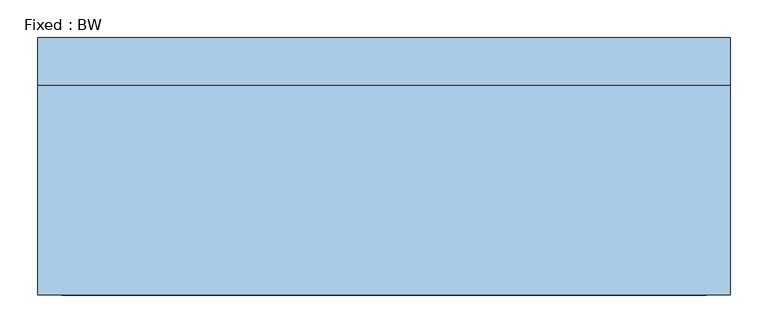
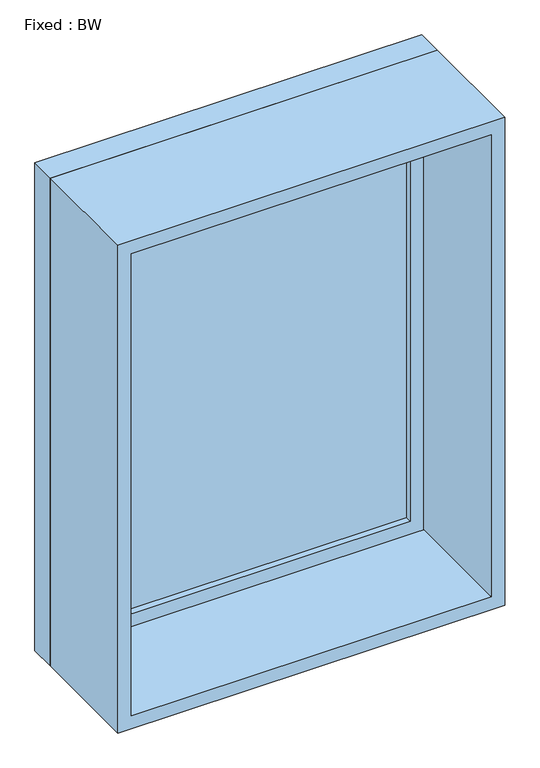
"""IFC4 building model written with IfcOpenShell, lengths in millimetres: window geometry, Fixed : BW."""

from ifc_helpers import new_model, si_unit, frame, origin, place, context, project, spatial, polyline, outline, extrude, source, transform, mapped, element, save


def fixed_bw_be0fa6e9(model_context):
    return source(origin(), model_context, "Body", "SweptSolid", [
        extrude(outline(polyline([(355.6, 122.4883569), (-431.8, 122.4883569), (-431.8, 135.1883569), (355.6, 135.1883569), (355.6, 122.4883569)])), frame((0.0, 0.0, 977.9), z_axis=(0.0, 0.0, 1.0), x_axis=(1.0, 0.0, 0.0)), (0.0, 0.0, 1.0), 1092.2),
        extrude(outline(polyline([(2114.55, -476.25), (933.45, -476.25), (933.45, 400.05), (2114.55, 400.05), (2114.55, -476.25)]), holes=[polyline([(2070.1, -431.8), (2070.1, 355.6), (977.9, 355.6), (977.9, -431.8), (2070.1, -431.8)])]), frame((0.0, 106.6133569, 0.0), z_axis=(0.0, 1.0, 0.0), x_axis=(0.0, 0.0, 1.0)), (0.0, 0.0, 1.0), 44.45),
        extrude(outline(polyline([(2133.6, -495.3), (914.4, -495.3), (914.4, 419.1), (2133.6, 419.1), (2133.6, -495.3)]), holes=[polyline([(2101.85, -463.55), (2101.85, 387.35), (946.15, 387.35), (946.15, -463.55), (2101.85, -463.55)])]), frame((0.0, -170.1133569, 0.0), z_axis=(0.0, 1.0, 0.0), x_axis=(0.0, 0.0, 1.0)), (0.0, 0.0, 1.0), 276.7267137),
        extrude(outline(polyline([(2133.6, 419.1), (2133.6, -495.3), (914.4, -495.3), (914.4, 419.1), (2133.6, 419.1)]), holes=[polyline([(2114.55, 400.05), (933.45, 400.05), (933.45, -476.25), (2114.55, -476.25), (2114.55, 400.05)])]), frame((0.0, 106.6133569, 0.0), z_axis=(0.0, 1.0, 0.0), x_axis=(0.0, 0.0, 1.0)), (0.0, 0.0, 1.0), 63.5),
    ])


if __name__ == "__main__":
    model = new_model("IFC4")
    model_context = context("Model", 3, world=origin())
    ifc_project = project(units=[si_unit("LENGTHUNIT", "METRE", prefix="MILLI")], contexts=[model_context])
    site = spatial("IfcSite", under=ifc_project)
    building = spatial("IfcBuilding", under=site)
    placement = place(None, origin())
    fixed_bw_shape = fixed_bw_be0fa6e9(model_context)
    element("IfcWindow", 1, ObjectType="Fixed : BW", at=placement, inside=building, context=model_context, shape_type="MappedRepresentation", body=[
        mapped(fixed_bw_shape, transform((0.0, 0.0, 0.0), x_axis=(1.0, 0.0, 0.0), y_axis=(0.0, 1.0, 0.0), z_axis=(0.0, 0.0, 1.0))),
    ])
    save(model, "model.ifc")

# Revit data of these elements
# Type "Fixed : BW"
#   Type Mark = "18"
#   Construction Type Id = "GSP4R"
#   Assembly Code = "B2020100"
#   Analytic Construction = "1/8 in Pilkington single glazing"
#   Visual Light Transmittance = 0.9
#   Solar Heat Gain Coefficient = 0.78
#   Heat Transfer Coefficient (U) = 0.6496 BTU/(h·ft²·°F)
#   Height = 4' - 0"
#   Default Sill Height = 3' - 0"
#   Width = 3' - 0"
#   Window Inset = 0' - 0 3/4"
#   Define Thermal Properties by = 1
#   Glass Pane Material = Glass
#   Sash Material = Sash
#   Wall Closure = (empty or 0)
# Element 1 (IfcWindow, "Fixed : BW")
#   Materials on its faces: "Sash", "Glass"
# Materials
#   "Glass": class "Glass", colour RGB 0 128 192, transparency 0.75, Description = "Soda Lime Glass", Cost = 0
#   "Sash": class "Wood", colour RGB 224 178 126, transparency 0, Cost = 0
